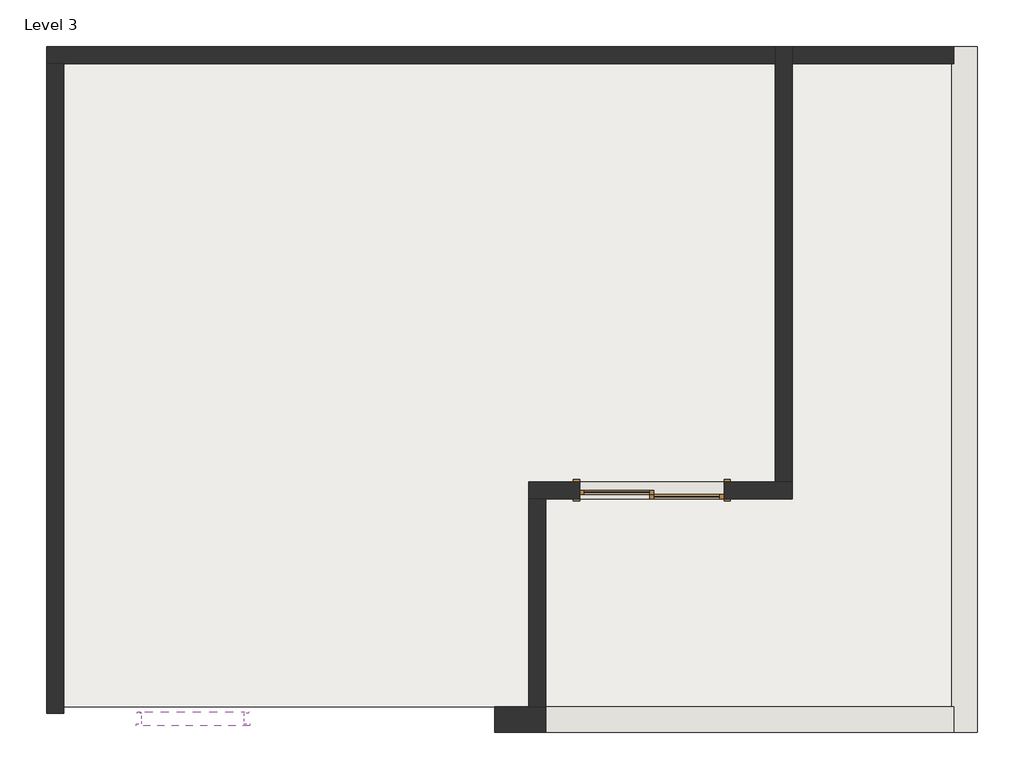
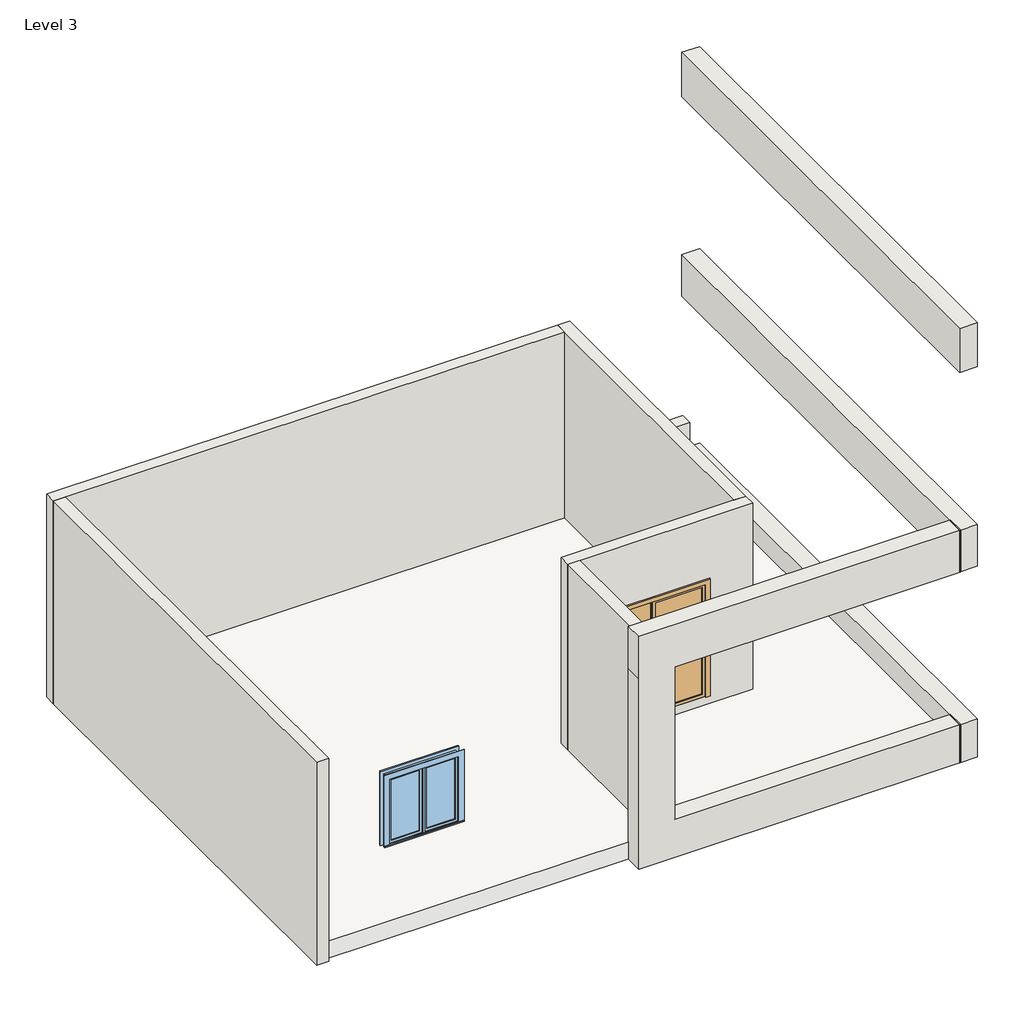
# One storey, incomplete: 8 walls, 1 door, 1 roof, 1 window.
"""IFC4 building model written with IfcOpenShell, lengths in millimetres."""

from ifc_helpers import new_model, si_unit, frame, origin, place, context, project, spatial, polyline, outline, extrude, faceted_brep, transform, mapped, element, save
from components import door_076b30e0, walls_2_walls_2_451c460c, walls_3_walls_3_273bb310, window_40d2abec

model = new_model("IFC4")

# Units and contexts
model_context = context("Model", 3, world=origin())
ifc_project = project(units=[si_unit("LENGTHUNIT", "METRE", prefix="MILLI")], contexts=[model_context])

# Site, building, storey
site = spatial("IfcSite", under=ifc_project)
building = spatial("IfcBuilding", under=site)
storey = spatial("IfcBuildingStorey", under=building, Name="Level 3", Elevation=7315.2)

# Door
placement = place(None, origin())
door_shape = door_076b30e0(model_context)
element("IfcDoor", 1, ObjectType="Door-Double-Sliding : 68\" x 80\"", at=placement, inside=storey, context=model_context, shape_type="MappedRepresentation", body=[
    mapped(door_shape, transform((-6976.7304753, 5777.4732783, 7772.4), x_axis=(-1.0, 0.0, 0.0), y_axis=(0.0, -1.0, 0.0), z_axis=(0.0, 0.0, 1.0))),
])

# Roof
element("IfcRoof", 2, ObjectType="Generic - 12\"", at=placement, inside=storey, context=model_context, shape_type="SweptSolid", body=[
    extrude(outline(polyline([(-14209.7864811, 10932.8297737), (-3389.3864811, 10932.8297737), (-3389.3864811, 3058.8297737), (-14209.7864811, 3058.8297737), (-14209.7864811, 10932.8297737)])), frame((0.0, 0.0, 7315.2), z_axis=(0.0, 0.0, 1.0), x_axis=(1.0, 0.0, 0.0)), (0.0, 0.0, 1.0), 304.8),
])

# Walls
element("IfcWall", 3, ObjectType="Generic - 8\"", at=placement, inside=storey, context=model_context, shape_type="Brep", body=[
    faceted_brep([(-5300.3304753, 5752.0732783, 7315.2), (-5503.5304753, 5752.0732783, 7315.2), (-8449.9304753, 5752.0732783, 7315.2), (-8449.9304753, 5752.0732783, 10972.8), (-5503.5304753, 5752.0732783, 10972.8), (-5300.3304753, 5752.0732783, 10972.8), (-6113.1304753, 5752.0732783, 9804.4), (-7840.3304753, 5752.0732783, 9804.4), (-7840.3304753, 5752.0732783, 7772.4), (-6113.1304753, 5752.0732783, 7772.4), (-5300.3304753, 5548.8732783, 7315.2), (-5300.3304753, 5548.8732783, 10972.8), (-8246.7304753, 5548.8732783, 10972.8), (-8449.9304753, 5548.8732783, 10972.8), (-8449.9304753, 5548.8732783, 7315.2), (-8246.7304753, 5548.8732783, 7315.2), (-6113.1304753, 5548.8732783, 9804.4), (-6113.1304753, 5548.8732783, 7772.4), (-7840.3304753, 5548.8732783, 7772.4), (-7840.3304753, 5548.8732783, 9804.4)], [[[0, 1, 2, 3, 4, 5], [6, 7, 8, 9]], [[10, 11, 12, 13, 14, 15], [16, 17, 18, 19]], [[2, 1, 0, 10, 15, 14]], [[5, 4, 3, 13, 12, 11]], [[3, 2, 14, 13]], [[0, 5, 11, 10]], [[17, 16, 6, 9]], [[18, 17, 9, 8]], [[19, 18, 8, 7]], [[16, 19, 7, 6]]]),
])
element("IfcWall", 4, ObjectType="Generic - 8\"", at=placement, inside=storey, context=model_context, shape_type="SweptSolid", body=[
    extrude(outline(polyline([(-8449.9304753, 3058.8297737), (-8449.9304753, 5548.8732783), (-8246.7304753, 5548.8732783), (-8246.7304753, 3058.8297737), (-8449.9304753, 3058.8297737)])), frame((0.0, 0.0, 7315.2), z_axis=(0.0, 0.0, 1.0), x_axis=(1.0, 0.0, 0.0)), (0.0, 0.0, 1.0), 3657.6),
])
element("IfcWall", 5, ObjectType="Generic - 8\"", at=placement, inside=storey, context=model_context, shape_type="Brep", body=[
    faceted_brep([(-5300.3304753, 5752.0732783, 7315.2), (-5300.3304753, 10958.2297737, 7315.2), (-5300.3304753, 10958.2297737, 7602.0125244), (-5300.3304753, 10958.2297737, 8590.8392493), (-5300.3304753, 10958.2297737, 10972.8), (-5300.3304753, 5752.0732783, 10972.8), (-5503.5304753, 5752.0732783, 7315.2), (-5503.5304753, 5752.0732783, 10972.8), (-5503.5304753, 10755.0297737, 10972.8), (-5503.5304753, 10958.2297737, 10972.8), (-5503.5304753, 10958.2297737, 7315.2), (-5503.5304753, 10755.0297737, 7315.2)], [[[0, 1, 2, 3, 4, 5]], [[6, 7, 8, 9, 10, 11]], [[1, 0, 6, 11, 10]], [[5, 4, 9, 8, 7]], [[0, 5, 7, 6]], [[1, 10, 9, 4, 3, 2]]]),
])
element("IfcWall", 6, ObjectType="Generic - 8\"", at=placement, inside=storey, context=model_context, shape_type="Brep", body=[
    faceted_brep([(-5503.5304753, 10958.2297737, 10972.8), (-5503.5304753, 10958.2297737, 7315.2), (-14212.6992777, 10958.2297737, 7315.2), (-14212.6992777, 10958.2297737, 10972.8), (-5503.5304753, 10755.0297737, 7315.2), (-5503.5304753, 10755.0297737, 10972.8), (-14009.4992777, 10755.0297737, 10972.8), (-14212.6992777, 10755.0297737, 10972.8), (-14212.6992777, 10755.0297737, 7315.2), (-14009.4992777, 10755.0297737, 7315.2)], [[[0, 1, 2, 3]], [[4, 5, 6, 7, 8, 9]], [[2, 1, 4, 9, 8]], [[0, 3, 7, 6, 5]], [[3, 2, 8, 7]], [[0, 5, 4, 1]]]),
])
element("IfcWall", 7, ObjectType="Generic - 8\"", at=placement, inside=storey, context=model_context, shape_type="SweptSolid", body=[
    extrude(outline(polyline([(-14212.6992777, 2982.6297737), (-14212.6992777, 10755.0297737), (-14009.4992777, 10755.0297737), (-14009.4992777, 2982.6297737), (-14212.6992777, 2982.6297737)])), frame((0.0, 0.0, 7315.2), z_axis=(0.0, 0.0, 1.0), x_axis=(1.0, 0.0, 0.0)), (0.0, 0.0, 1.0), 3657.6),
])
element("IfcWall", 8, ObjectType="Generic - 8\"", at=placement, inside=storey, context=model_context, shape_type="SweptSolid", body=[
    extrude(outline(polyline([(-3369.9304753, 10755.0297737), (-5300.3304753, 10755.0297737), (-5300.3304753, 10958.2297737), (-3369.9304753, 10958.2297737), (-3369.9304753, 10755.0297737)])), frame((0.0, 0.0, 7602.0125244), z_axis=(0.0, 0.0, 1.0), x_axis=(1.0, 0.0, 0.0)), (0.0, 0.0, 1.0), 988.8267249),
])
walls_2_walls_2_shape = walls_2_walls_2_451c460c(model_context)
element("IfcWall", 9, ObjectType="Walls 2 : Walls 2", at=placement, inside=storey, context=model_context, shape_type="MappedRepresentation", body=[
    mapped(walls_2_walls_2_shape, transform((0.0, 0.0, 0.0), x_axis=(1.0, 0.0, 0.0), y_axis=(0.0, 1.0, 0.0), z_axis=(0.0, 0.0, 1.0))),
])
walls_3_walls_3_shape = walls_3_walls_3_273bb310(model_context)
element("IfcWall", 10, ObjectType="Walls 3 : Walls 3", at=placement, inside=storey, context=model_context, shape_type="MappedRepresentation", body=[
    mapped(walls_3_walls_3_shape, transform((0.0, 0.0, 0.0), x_axis=(1.0, 0.0, 0.0), y_axis=(0.0, 1.0, 0.0), z_axis=(0.0, 0.0, 1.0))),
])

# Window
window_shape = window_40d2abec(model_context)
element("IfcWindow", 11, ObjectType="Casement Dbl with Trim.0001 : 48\" x 48\"", at=placement, inside=storey, context=model_context, shape_type="MappedRepresentation", body=[
    mapped(window_shape, transform((-12463.1304753, 2938.1797737, 8236.8437858), x_axis=(-1.0, 0.0, 0.0), y_axis=(0.0, -1.0, 0.0), z_axis=(0.0, 0.0, 1.0))),
])

save(model, "model.ifc")

# Revit data of these elements
# Type "Door-Double-Sliding : 68\" x 80\""
#   Type Mark = "8"
#   Construction Type Id = "opn-d45"
#   Assembly Code = "C1020"
#   Analytic Construction = "Wood frame, double glass door "
#   Thickness = 0' - 2"
#   Thermal Resistance (R) = 1.8150 (h·ft²·°F)/BTU
#   Heat Transfer Coefficient (U) = 0.5510 BTU/(h·ft²·°F)
#   Height = 6' - 8"
#   Rail Width = 0' - 2"
#   Stiles = 0' - 2"
#   Trim Projection Ext = 0' - 1"
#   Trim Projection Int = 0' - 1"
#   Trim Width = 0' - 3"
#   Width = 5' - 8"
#   Define Thermal Properties by = 1
#   Glazing = Glass
#   Panel Material = Wood - Birch - Solid Stained Light Low Gloss
#   Trim Material = Paint - Sienna
#   Visual Light Transmittance = 0
#   Solar Heat Gain Coefficient = 0
#   Function = (empty or 0)
#   Wall Closure = (empty or 0)
# Type "Generic - 12\""
#   Assembly Code = "B1020"
#   Layers, outside or top first: 1' - 0" no material (function 1)
# Type "Generic - 8\""
#   Assembly Code = "B2010"
#   Layers, outside or top first: 0' - 8" no material (function 1)
# Type "Casement Dbl with Trim.0001 : 48\" x 48\""
#   Type Mark = "10"
#   Construction Type Id = "GSP4R"
#   Assembly Code = "B2020100"
#   Analytic Construction = "1/8 in Pilkington single glazing"
#   Visual Light Transmittance = 0.9
#   Solar Heat Gain Coefficient = 0.78
#   Heat Transfer Coefficient (U) = 0.6496 BTU/(h·ft²·°F)
#   Height = 4' - 0"
#   Default Sill Height = 3' - 0"
#   Trim Projection - Ext. = 0' - 0 1/2"
#   Trim Projection - Int. = 0' - 0 3/4"
#   Trim Width - Exterior = 0' - 3 1/2"
#   Trim Width - Interior = 0' - 3 1/2"
#   Width = 4' - 0"
#   Window Inset = 0' - 0 3/4"
#   Define Thermal Properties by = 1
#   Glass Pane Material = Glass
#   Sash Material = Sash
#   Trim Exterior Material = Trim
#   Trim Interior Material = Trim
#   Wall Closure = (empty or 0)
# Element 1 (IfcDoor, "Door-Double-Sliding : 68\" x 80\"")
#   Phase Created = New Construction
#   Materials on its faces: "Paint - Sienna", "Wood - Birch - Solid Stained Light Low Gloss", "Glass"
# Element 2 (IfcRoof, "Generic - 12\"")
#   built-in parameter 1001705 = 25 (stored number, unit not read)
#   built-in parameter 1001710 = 33615
#   Phase Created = New Construction
#   Materials on its faces: "Default Roof"
# Elements 3, 4, 5, 6, 7 (IfcWall, "Generic - 8\"")
#   Top Offset = 0' - 0"
#   Base Offset = 0' - 0"
#   Unconnected Height = 12' - 0"
#   wall height = 12' - 0"
#   Phase Created = New Construction
#   Base Constraint = Level 3
#   Materials on its faces: "Default Wall"
# Element 8 (IfcWall, "Generic - 8\"")
#   built-in parameter 1001111 = 0' - 11.29183"
#   Top Offset = 0' - 0"
#   Base Offset = 0' - 11.29183"
#   Unconnected Height = 3' - 2.93019"
#   wall height = 3' - 2.93019"
#   Phase Created = New Construction
#   Base Constraint = Level 3
#   Materials on its faces: "Default Wall"
# Element 9 (IfcWall, "Walls 2 : Walls 2")
#   Phase Created = New Construction
#   Materials on its faces: "Default Wall"
# Element 10 (IfcWall, "Walls 3 : Walls 3")
#   Phase Created = New Construction
#   Materials on its faces: "Default Wall"
# Element 11 (IfcWindow, "Casement Dbl with Trim.0001 : 48\" x 48\"")
#   Mark = "4"
#   Phase Created = New Construction
#   Materials on its faces: "Sash", "Trim", "Glass"
# Materials
#   "Glass": class "Glass", colour RGB 0 128 192, transparency 0.75, Description = "Soda Lime Glass", Cost = 0
#   "Wood - Birch - Solid Stained Light Low Gloss": class "Wood", colour RGB 210 159 95, transparency 0, Cost = 0
#   "Paint - Sienna": colour RGB 118 70 51, transparency 0, Cost = 0
#   "Sash": class "Wood", colour RGB 224 178 126, transparency 0
#   "Trim": class "Wood", colour RGB 224 178 126, transparency 0
#   "Default Roof": colour RGB 88 101 114, transparency 0
#   "Default Wall": colour RGB 128 128 128, transparency 0
